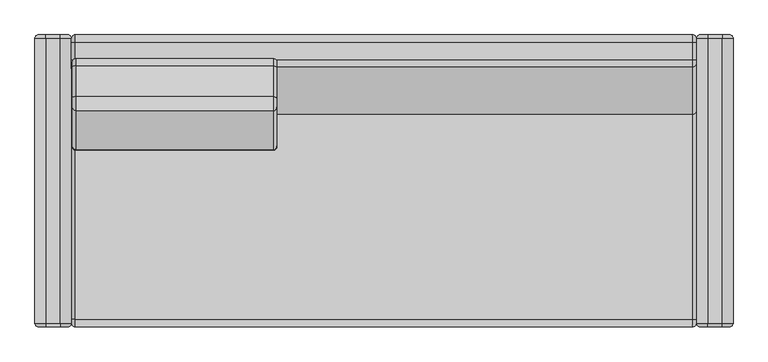
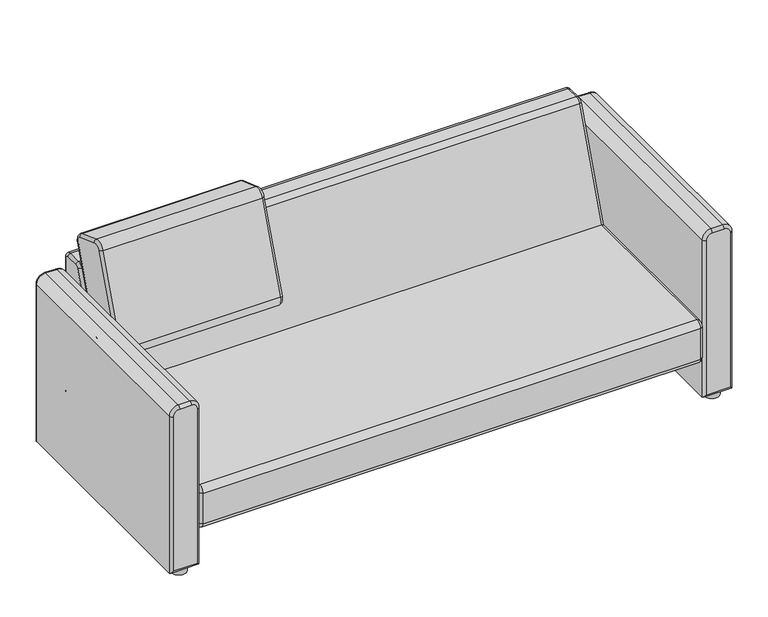
"""IFC4 building model written with IfcOpenShell, lengths in millimetres: furniture geometry."""

from ifc_helpers import new_model, si_unit, point, frame, frame_2d, origin, origin_with_axes, place, context, project, spatial, circle_curve, ellipse_curve, trimmed, segment, composite_curve, outline, extrude, source, transform, mapped, element, save
from ifc_brep_helpers import plane_surface, cylinder_surface, revolved_surface, advanced_brep


def furniture_2fc85b74(model_context):
    return source(origin(), model_context, "Body", "SolidModel", [
        advanced_brep(
        [(-945.0, 0.0, 590.0), (-945.0, 0.0, 35.0), (-865.0, 0.0, 35.0), (-865.0, 0.0, 590.0), (-885.0, 0.0, 610.0), (-925.0, 0.0, 610.0), (-865.0, 800.0, 590.0), (-865.0, 800.0, 35.0), (-945.0, 800.0, 35.0), (-945.0, 800.0, 590.0), (-925.0, 800.0, 610.0), (-885.0, 800.0, 610.0), (-855.0, 9.9999877, 590.0), (-855.0, 790.0000093, 590.0), (-885.0, 790.0, 620.0), (-885.0, 10.0, 620.0), (-925.0, 9.9999878, 620.0), (-925.0, 790.0, 620.0), (-955.0, 790.0, 590.0), (-955.0, 9.9999878, 590.0), (-855.0, 10.0, 25.0), (-855.0, 790.0, 25.0), (-955.0, 10.0, 25.0), (-955.0, 790.0, 25.0)],
        [
            (0, 1),
            (1, 2),
            (2, 3),
            (3, 4, circle_curve(frame((-885.0, 0.0, 590.0), z_axis=(0.0, -1.0, 0.0), x_axis=(0.0, 0.0, 1.0)), 20.0)),
            (4, 5),
            (5, 0, circle_curve(frame((-925.0, 0.0, 590.0), z_axis=(0.0, -1.0, 0.0), x_axis=(-1.0, 0.0, 0.0)), 20.0)),
            (6, 7),
            (7, 8),
            (8, 9),
            (9, 10, circle_curve(frame((-925.0, 800.0, 590.0), z_axis=(0.0, 1.0, 0.0), x_axis=(0.0, 0.0, 1.0)), 20.0)),
            (10, 11),
            (11, 6, circle_curve(frame((-885.0, 800.0, 590.0), z_axis=(0.0, 1.0, 0.0), x_axis=(1.0, 0.0, 0.0)), 20.0)),
            (12, 13),
            (13, 14, circle_curve(frame((-885.0, 790.0, 590.0), z_axis=(0.0, -1.0, 0.0), x_axis=(-1.0, 0.0, 0.0)), 30.0)),
            (14, 15),
            (15, 12, circle_curve(frame((-885.0, 10.0, 590.0), z_axis=(0.0, 1.0, 0.0), x_axis=(-1.0, 0.0, 0.0)), 30.0)),
            (16, 17),
            (17, 18, circle_curve(frame((-925.0, 790.0, 590.0), z_axis=(0.0, -1.0, 0.0), x_axis=(-1.0, 0.0, 0.0)), 30.0)),
            (18, 19),
            (19, 16, circle_curve(frame((-925.0, 10.0, 590.0), z_axis=(0.0, 1.0, 0.0), x_axis=(-1.0, 0.0, 0.0)), 30.0)),
            (20, 21),
            (21, 13),
            (12, 20),
            (22, 23),
            (23, 21),
            (20, 22),
            (18, 23),
            (22, 19),
            (14, 17),
            (16, 15),
            (19, 0, circle_curve(frame((-945.0, 10.0, 590.0), z_axis=(0.0, 0.0, 1.0), x_axis=(-1.0, 0.0, 0.0)), 10.0)),
            (5, 16, circle_curve(frame((-925.0, 10.0, 610.0), z_axis=(-1.0, 0.0, 0.0), x_axis=(0.0, 0.0, 1.0)), 10.0)),
            (4, 15, circle_curve(frame((-885.0, 10.0, 610.0), z_axis=(-1.0, 0.0, 0.0), x_axis=(0.0, 0.0, 1.0)), 10.0)),
            (3, 12, circle_curve(frame((-865.0, 10.0, 590.0), z_axis=(0.0, 0.0, 1.0), x_axis=(1.0, 0.0, 0.0)), 10.0)),
            (2, 20, ellipse_curve(frame((-865.0, 10.0, 35.0), z_axis=(0.7071067811865458, 0.0, 0.7071067811865492), x_axis=(0.7071067811865492, 0.0, -0.7071067811865458)), 14.1421356, 10.0)),
            (1, 22, ellipse_curve(frame((-945.0, 10.0, 35.0), z_axis=(0.7071067811865492, 0.0, -0.7071067811865457), x_axis=(-0.707106781186546, 0.0, -0.7071067811865491)), 14.1421356, 10.0)),
            (13, 6, circle_curve(frame((-865.0, 790.0, 590.0), z_axis=(0.0, 0.0, 1.0), x_axis=(-1.0, 0.0, 0.0)), 10.0)),
            (11, 14, circle_curve(frame((-885.0, 790.0, 610.0), z_axis=(1.0, 0.0, 0.0), x_axis=(0.0, 0.0, -1.0)), 10.0)),
            (10, 17, circle_curve(frame((-925.0, 790.0, 610.0), z_axis=(1.0, 0.0, 0.0), x_axis=(0.0, 0.0, -1.0)), 10.0)),
            (9, 18, circle_curve(frame((-945.0, 790.0, 590.0), z_axis=(0.0, 0.0, 1.0), x_axis=(1.0, 0.0, 0.0)), 10.0)),
            (8, 23, ellipse_curve(frame((-945.0, 790.0, 35.0), z_axis=(-0.7071067811865492, 0.0, 0.7071067811865458), x_axis=(-0.7071067811865457, 0.0, -0.7071067811865492)), 14.1421356, 10.0)),
            (7, 21, ellipse_curve(frame((-865.0, 790.0, 35.0), z_axis=(-0.707106781186546, 0.0, -0.7071067811865491), x_axis=(0.707106781186549, 0.0, -0.707106781186546)), 14.1421356, 10.0)),
        ],
        [
            plane_surface(frame((-915.0, 0.0, 590.0), z_axis=(0.0, -1.0, 0.0), x_axis=(0.0, 0.0, 1.0))),
            plane_surface(frame((-915.0, 800.0, 590.0), z_axis=(0.0, 1.0, 0.0), x_axis=(0.0, 0.0, -1.0))),
            cylinder_surface(frame((-885.0, 800.0, 590.0), z_axis=(0.0, -1.0, 0.0), x_axis=(-1.0, 0.0, 0.0)), 30.0),
            cylinder_surface(frame((-925.0, 800.0, 590.0), z_axis=(0.0, -1.0, 0.0), x_axis=(-1.0, 0.0, 0.0)), 30.0),
            plane_surface(frame((-855.0, 0.0, 590.0), z_axis=(1.0, 0.0, 0.0), x_axis=(0.0, 1.0, 0.0))),
            plane_surface(frame((-855.0, 0.0, 25.0), z_axis=(0.0, 0.0, -1.0), x_axis=(0.0, 1.0, 0.0))),
            plane_surface(frame((-955.0, 0.0, 25.0), z_axis=(-1.0, 0.0, 0.0), x_axis=(0.0, 1.0, 0.0))),
            plane_surface(frame((-925.0, 0.0, 620.0), z_axis=(0.0, 0.0, 1.0), x_axis=(0.0, 1.0, 0.0))),
            revolved_surface(trimmed(ellipse_curve(frame((-945.0, 10.0, 590.0), z_axis=(0.0, 0.0, 1.0), x_axis=(-1.0, 0.0, 0.0)), 10.0, 10.0), [point((-955.0, 10.0, 590.0))], [point((-945.0, 0.0, 590.0))], True, "CARTESIAN"), (-925.0, 0.0, 590.0), (0.0, -1.0, 0.0)),
            cylinder_surface(frame((-925.0, 10.0, 610.0), z_axis=(1.0, 0.0, 0.0), x_axis=(0.0, 0.0, 1.0)), 10.0),
            revolved_surface(trimmed(ellipse_curve(frame((-885.0, 10.0, 610.0), z_axis=(1.0, 0.0, 0.0), x_axis=(0.0, 0.0, 1.0)), 10.0, 10.0), [point((-885.0, 10.0, 620.0))], [point((-885.0, 0.0, 610.0))], True, "CARTESIAN"), (-885.0, 0.0, 590.0), (0.0, -1.0, 0.0)),
            cylinder_surface(frame((-865.0, 10.0, 590.0), z_axis=(0.0, 0.0, -1.0), x_axis=(1.0, 0.0, 0.0)), 10.0),
            cylinder_surface(frame((-855.0, 10.0, 35.0), z_axis=(-1.0, 0.0, 0.0), x_axis=(0.0, 0.0, -1.0)), 10.0),
            cylinder_surface(frame((-945.0, 10.0, 25.0), z_axis=(0.0, 0.0, 1.0), x_axis=(-1.0, 0.0, 0.0)), 10.0),
            revolved_surface(trimmed(ellipse_curve(frame((-865.0, 790.0, 590.0), z_axis=(0.0, 0.0, 1.0), x_axis=(-1.0, 0.0, 0.0)), 10.0, 10.0), [point((-855.0, 790.0, 590.0))], [point((-865.0, 800.0, 590.0))], True, "CARTESIAN"), (-885.0, 800.0, 590.0), (0.0, 1.0, 0.0)),
            cylinder_surface(frame((-885.0, 790.0, 610.0), z_axis=(-1.0, 0.0, 0.0), x_axis=(0.0, 0.0, -1.0)), 10.0),
            revolved_surface(trimmed(ellipse_curve(frame((-925.0, 790.0, 610.0), z_axis=(-1.0, 0.0, 0.0), x_axis=(0.0, 0.0, -1.0)), 10.0, 10.0), [point((-925.0, 790.0, 620.0))], [point((-925.0, 800.0, 610.0))], True, "CARTESIAN"), (-925.0, 800.0, 590.0), (0.0, 1.0, 0.0)),
            cylinder_surface(frame((-945.0, 790.0, 590.0), z_axis=(0.0, 0.0, -1.0), x_axis=(1.0, 0.0, 0.0)), 10.0),
            cylinder_surface(frame((-955.0, 790.0, 35.0), z_axis=(1.0, 0.0, 0.0), x_axis=(0.0, 0.0, 1.0)), 10.0),
            cylinder_surface(frame((-865.0, 790.0, 25.0), z_axis=(0.0, 0.0, 1.0), x_axis=(-1.0, 0.0, 0.0)), 10.0),
        ],
        [
            (0, [[1, 2, 3, 4, 5, 6]]),
            (1, [[7, 8, 9, 10, 11, 12]]),
            (2, [[13, 14, 15, 16]]),
            (3, [[17, 18, 19, 20]]),
            (4, [[21, 22, -13, 23]]),
            (5, [[24, 25, -21, 26]]),
            (6, [[-19, 27, -24, 28]]),
            (7, [[-15, 29, -17, 30]]),
            (8, [[-20, 31, -6, 32]]),
            (9, [[-5, 33, -30, -32]]),
            (10, [[-4, 34, -16, -33]]),
            (11, [[-3, 35, -23, -34]]),
            (12, [[-2, 36, -26, -35]]),
            (13, [[-28, -36, -1, -31]]),
            (14, [[-14, 37, -12, 38]]),
            (15, [[-11, 39, -29, -38]]),
            (16, [[-10, 40, -18, -39]]),
            (17, [[-9, 41, -27, -40]]),
            (18, [[-8, 42, -25, -41]]),
            (19, [[-22, -42, -7, -37]]),
        ],
    ),
        extrude(outline(composite_curve([segment(trimmed(circle_curve(frame_2d((-905.0, 760.0)), 25.0), [point((-880.0, 760.0))], [point((-930.0, 760.0))], False, "CARTESIAN"), True, "CONTINUOUS"), segment(trimmed(circle_curve(frame_2d((-905.0, 760.0)), 25.0), [point((-930.0, 760.0))], [point((-880.0, 760.0))], False, "CARTESIAN"), True, "CONTINUOUS")], self_intersect=False)), origin_with_axes(), (0.0, 0.0, 1.0), 25.0),
        extrude(outline(composite_curve([segment(trimmed(circle_curve(frame_2d((-905.0, 40.0)), 25.0), [point((-880.0, 40.0))], [point((-930.0, 40.0))], False, "CARTESIAN"), True, "CONTINUOUS"), segment(trimmed(circle_curve(frame_2d((-905.0, 40.0)), 25.0), [point((-930.0, 40.0))], [point((-880.0, 40.0))], False, "CARTESIAN"), True, "CONTINUOUS")], self_intersect=False)), origin_with_axes(), (0.0, 0.0, 1.0), 25.0),
        advanced_brep(
        [(946.1853865, 0.0, 590.0), (926.1853865, 0.0, 610.0), (886.1853865, 0.0, 610.0), (866.1853865, 0.0, 590.0), (866.1853865, 0.0, 35.0), (946.1853865, 0.0, 35.0), (866.1853865, 800.0, 590.0), (886.1853865, 800.0, 610.0), (926.1853865, 800.0, 610.0), (946.1853865, 800.0, 590.0), (946.1853865, 800.0, 35.0), (866.1853865, 800.0, 35.0), (856.1853865, 10.0, 590.0), (886.1853865, 10.0, 620.0), (886.1853865, 790.000012, 620.0), (856.1853865, 790.0, 590.0), (926.1853865, 10.0, 620.0), (956.1853865, 10.0, 590.0), (956.1853865, 790.0000092, 590.0), (926.1853865, 790.0, 620.0), (856.1853865, 10.0, 25.0), (856.1853865, 790.0, 25.0), (956.1853865, 10.0, 25.0), (956.1853865, 790.0, 25.0)],
        [
            (0, 1, circle_curve(frame((926.1853865, 0.0, 590.0), z_axis=(0.0, -1.0, 0.0), x_axis=(1.0, 0.0, 0.0)), 20.0)),
            (1, 2),
            (2, 3, circle_curve(frame((886.1853865, 0.0, 590.0), z_axis=(0.0, -1.0, 0.0), x_axis=(0.0, 0.0, 1.0)), 20.0)),
            (3, 4),
            (4, 5),
            (5, 0),
            (6, 7, circle_curve(frame((886.1853865, 800.0, 590.0), z_axis=(0.0, 1.0, 0.0), x_axis=(-1.0, 0.0, 0.0)), 20.0)),
            (7, 8),
            (8, 9, circle_curve(frame((926.1853865, 800.0, 590.0), z_axis=(0.0, 1.0, 0.0), x_axis=(0.0, 0.0, 1.0)), 20.0)),
            (9, 10),
            (10, 11),
            (11, 6),
            (12, 13, circle_curve(frame((886.1853865, 10.0, 590.0), z_axis=(0.0, 1.0, 0.0), x_axis=(1.0, 0.0, 0.0)), 30.0)),
            (13, 14),
            (14, 15, circle_curve(frame((886.1853865, 790.0, 590.0), z_axis=(0.0, -1.0, 0.0), x_axis=(1.0, 0.0, 0.0)), 30.0)),
            (15, 12),
            (16, 17, circle_curve(frame((926.1853865, 10.0, 590.0), z_axis=(0.0, 1.0, 0.0), x_axis=(1.0, 0.0, 0.0)), 30.0)),
            (17, 18),
            (18, 19, circle_curve(frame((926.1853865, 790.0, 590.0), z_axis=(0.0, -1.0, 0.0), x_axis=(1.0, 0.0, 0.0)), 30.0)),
            (19, 16),
            (20, 12),
            (15, 21),
            (21, 20),
            (22, 20),
            (21, 23),
            (23, 22),
            (17, 22),
            (23, 18),
            (13, 16),
            (19, 14),
            (16, 1, circle_curve(frame((926.1853865, 10.0, 610.0), z_axis=(1.0, 0.0, 0.0), x_axis=(0.0, 0.0, 1.0)), 10.0)),
            (0, 17, circle_curve(frame((946.1853865, 10.0, 590.0), z_axis=(0.0, 0.0, 1.0), x_axis=(1.0, 0.0, 0.0)), 10.0)),
            (13, 2, circle_curve(frame((886.1853865, 10.0, 610.0), z_axis=(1.0, 0.0, 0.0), x_axis=(0.0, 0.0, 1.0)), 10.0)),
            (12, 3, circle_curve(frame((866.1853865, 10.0, 590.0), z_axis=(0.0, 0.0, 1.0), x_axis=(-1.0, 0.0, 0.0)), 10.0)),
            (20, 4, ellipse_curve(frame((866.1853865, 10.0, 35.0), z_axis=(-0.7071067811865458, 0.0, 0.7071067811865492), x_axis=(-0.7071067811865492, 0.0, -0.7071067811865458)), 14.1421356, 10.0)),
            (22, 5, ellipse_curve(frame((946.1853865, 10.0, 35.0), z_axis=(-0.7071067811865492, 0.0, -0.7071067811865457), x_axis=(0.707106781186546, 0.0, -0.7071067811865491)), 14.1421356, 10.0)),
            (14, 7, circle_curve(frame((886.1853865, 790.0, 610.0), z_axis=(-1.0, 0.0, 0.0), x_axis=(0.0, 0.0, -1.0)), 10.0)),
            (6, 15, circle_curve(frame((866.1853865, 790.0, 590.0), z_axis=(0.0, 0.0, 1.0), x_axis=(1.0, 0.0, 0.0)), 10.0)),
            (19, 8, circle_curve(frame((926.1853865, 790.0, 610.0), z_axis=(-1.0, 0.0, 0.0), x_axis=(0.0, 0.0, -1.0)), 10.0)),
            (18, 9, circle_curve(frame((946.1853865, 790.0, 590.0), z_axis=(0.0, 0.0, 1.0), x_axis=(-1.0, 0.0, 0.0)), 10.0)),
            (23, 10, ellipse_curve(frame((946.1853865, 790.0, 35.0), z_axis=(0.7071067811865492, 0.0, 0.7071067811865458), x_axis=(0.7071067811865457, 0.0, -0.7071067811865492)), 14.1421356, 10.0)),
            (21, 11, ellipse_curve(frame((866.1853865, 790.0, 35.0), z_axis=(0.707106781186546, 0.0, -0.7071067811865491), x_axis=(-0.707106781186549, 0.0, -0.707106781186546)), 14.1421356, 10.0)),
        ],
        [
            plane_surface(frame((916.1853865, 0.0, 590.0), z_axis=(0.0, -1.0, 0.0), x_axis=(0.0, 0.0, 1.0))),
            plane_surface(frame((916.1853865, 800.0, 590.0), z_axis=(0.0, 1.0, 0.0), x_axis=(0.0, 0.0, -1.0))),
            cylinder_surface(frame((886.1853865, 800.0, 590.0), z_axis=(0.0, -1.0, 0.0), x_axis=(1.0, 0.0, 0.0)), 30.0),
            cylinder_surface(frame((926.1853865, 800.0, 590.0), z_axis=(0.0, -1.0, 0.0), x_axis=(1.0, 0.0, 0.0)), 30.0),
            plane_surface(frame((856.1853865, 0.0, 590.0), z_axis=(-1.0, 0.0, 0.0), x_axis=(0.0, 1.0, 0.0))),
            plane_surface(frame((856.1853865, 0.0, 25.0), z_axis=(0.0, 0.0, -1.0), x_axis=(0.0, 1.0, 0.0))),
            plane_surface(frame((956.1853865, 0.0, 25.0), z_axis=(1.0, 0.0, 0.0), x_axis=(0.0, 1.0, 0.0))),
            plane_surface(frame((926.1853865, 0.0, 620.0), z_axis=(0.0, 0.0, 1.0), x_axis=(0.0, 1.0, 0.0))),
            revolved_surface(trimmed(ellipse_curve(frame((946.1853865, 10.0, 590.0), z_axis=(0.0, 0.0, -1.0), x_axis=(1.0, 0.0, 0.0)), 10.0, 10.0), [point((956.1853865, 10.0, 590.0))], [point((946.1853865, 0.0, 590.0))], True, "CARTESIAN"), (926.1853865, 0.0, 590.0), (0.0, -1.0, 0.0)),
            cylinder_surface(frame((926.1853865, 10.0, 610.0), z_axis=(-1.0, 0.0, 0.0), x_axis=(0.0, 0.0, 1.0)), 10.0),
            revolved_surface(trimmed(ellipse_curve(frame((886.1853865, 10.0, 610.0), z_axis=(1.0, 0.0, 0.0), x_axis=(0.0, 0.0, 1.0)), 10.0, 10.0), [point((886.1853865, 10.0, 620.0))], [point((886.1853865, 0.0, 610.0))], True, "CARTESIAN"), (886.1853865, 0.0, 590.0), (0.0, -1.0, 0.0)),
            cylinder_surface(frame((866.1853865, 10.0, 590.0), z_axis=(0.0, 0.0, -1.0), x_axis=(-1.0, 0.0, 0.0)), 10.0),
            cylinder_surface(frame((856.1853865, 10.0, 35.0), z_axis=(1.0, 0.0, 0.0), x_axis=(0.0, 0.0, -1.0)), 10.0),
            cylinder_surface(frame((946.1853865, 10.0, 25.0), z_axis=(0.0, 0.0, 1.0), x_axis=(1.0, 0.0, 0.0)), 10.0),
            revolved_surface(trimmed(ellipse_curve(frame((866.1853865, 790.0, 590.0), z_axis=(0.0, 0.0, -1.0), x_axis=(1.0, 0.0, 0.0)), 10.0, 10.0), [point((856.1853865, 790.0, 590.0))], [point((866.1853865, 800.0, 590.0))], True, "CARTESIAN"), (886.1853865, 800.0, 590.0), (0.0, 1.0, 0.0)),
            cylinder_surface(frame((886.1853865, 790.0, 610.0), z_axis=(1.0, 0.0, 0.0), x_axis=(0.0, 0.0, -1.0)), 10.0),
            revolved_surface(trimmed(ellipse_curve(frame((926.1853865, 790.0, 610.0), z_axis=(-1.0, 0.0, 0.0), x_axis=(0.0, 0.0, -1.0)), 10.0, 10.0), [point((926.1853865, 790.0, 620.0))], [point((926.1853865, 800.0, 610.0))], True, "CARTESIAN"), (926.1853865, 800.0, 590.0), (0.0, 1.0, 0.0)),
            cylinder_surface(frame((946.1853865, 790.0, 590.0), z_axis=(0.0, 0.0, -1.0), x_axis=(-1.0, 0.0, 0.0)), 10.0),
            cylinder_surface(frame((956.1853865, 790.0, 35.0), z_axis=(-1.0, 0.0, 0.0), x_axis=(0.0, 0.0, 1.0)), 10.0),
            cylinder_surface(frame((866.1853865, 790.0, 25.0), z_axis=(0.0, 0.0, 1.0), x_axis=(1.0, 0.0, 0.0)), 10.0),
        ],
        [
            (0, [[1, 2, 3, 4, 5, 6]]),
            (1, [[7, 8, 9, 10, 11, 12]]),
            (2, [[13, 14, 15, 16]]),
            (3, [[17, 18, 19, 20]]),
            (4, [[21, -16, 22, 23]]),
            (5, [[24, -23, 25, 26]]),
            (6, [[27, -26, 28, -18]]),
            (7, [[29, -20, 30, -14]]),
            (8, [[31, -1, 32, -17]]),
            (9, [[-31, -29, 33, -2]]),
            (10, [[-33, -13, 34, -3]]),
            (11, [[-34, -21, 35, -4]]),
            (12, [[-35, -24, 36, -5]]),
            (13, [[-32, -6, -36, -27]]),
            (14, [[37, -7, 38, -15]]),
            (15, [[-37, -30, 39, -8]]),
            (16, [[-39, -19, 40, -9]]),
            (17, [[-40, -28, 41, -10]]),
            (18, [[-41, -25, 42, -11]]),
            (19, [[-38, -12, -42, -22]]),
        ],
    ),
        extrude(outline(composite_curve([segment(trimmed(circle_curve(frame_2d((906.1853865, 760.0)), 25.0), [point((881.1853865, 760.0))], [point((931.1853865, 760.0))], False, "CARTESIAN"), True, "CONTINUOUS"), segment(trimmed(circle_curve(frame_2d((906.1853865, 760.0)), 25.0), [point((931.1853865, 760.0))], [point((881.1853865, 760.0))], False, "CARTESIAN"), True, "CONTINUOUS")], self_intersect=False)), origin_with_axes(), (0.0, 0.0, 1.0), 25.0),
        extrude(outline(composite_curve([segment(trimmed(circle_curve(frame_2d((906.1853865, 40.0)), 25.0), [point((881.1853865, 40.0))], [point((931.1853865, 40.0))], False, "CARTESIAN"), True, "CONTINUOUS"), segment(trimmed(circle_curve(frame_2d((906.1853865, 40.0)), 25.0), [point((931.1853865, 40.0))], [point((881.1853865, 40.0))], False, "CARTESIAN"), True, "CONTINUOUS")], self_intersect=False)), origin_with_axes(), (0.0, 0.0, 1.0), 25.0),
        advanced_brep(
        [(855.0, 731.2835554, 660.0), (855.0, 721.8866292, 653.4202014), (855.0, 589.6124934, 290.0), (855.0, 20.0, 290.0), (855.0, 10.0, 280.0), (855.0, 10.0, 170.0), (855.0, 20.0, 160.0), (855.0, 780.0, 160.0), (855.0, 790.0, 170.0), (855.0, 790.0, 650.0), (855.0, 780.0, 660.0), (-855.0, 780.0, 660.0), (-855.0, 790.0, 650.0), (-855.0, 790.0, 170.0), (-855.0, 780.0, 160.0), (-855.0, 20.0, 160.0), (-855.0, 10.0, 170.0), (-855.0, 10.0, 280.0), (-855.0, 20.0, 290.0), (-855.0, 589.6124934, 290.0), (-855.0, 721.8866292, 653.4202014), (-855.0, 731.2835554, 660.0), (-845.0, 731.2835554, 670.0), (-845.0, 712.489703, 656.8404029), (845.0000088, 712.489703, 656.8404029), (845.0, 731.2835554, 670.0), (-845.0, 582.610418, 300.0), (845.0, 582.610418, 300.0), (-845.0, 20.0, 300.0), (845.0, 20.0, 300.0), (-845.0, 0.0, 280.0), (845.000009, 0.0, 280.0), (-845.0, 0.0, 170.0), (845.0, 0.0, 170.0), (-845.0, 20.0, 150.0), (845.000009, 20.0, 150.0), (-845.0, 780.0, 150.0), (845.0, 780.0, 150.0), (-845.0, 800.0, 170.0), (845.000009, 800.0, 170.0), (-845.0, 800.0, 650.0), (845.0, 800.0, 650.0), (-845.0, 780.0, 670.0), (845.0000092, 780.0, 670.0)],
        [
            (0, 1, circle_curve(frame((855.0, 731.2835554, 650.0), z_axis=(1.0, 0.0, 0.0), x_axis=(0.0, 0.0, 1.0)), 10.0)),
            (1, 2),
            (2, 3),
            (3, 4, circle_curve(frame((855.0, 20.0, 280.0), z_axis=(1.0, 0.0, 0.0), x_axis=(0.0, 0.0, 1.0)), 10.0)),
            (4, 5),
            (5, 6, circle_curve(frame((855.0, 20.0, 170.0), z_axis=(1.0, 0.0, 0.0), x_axis=(0.0, -1.0, 0.0)), 10.0)),
            (6, 7),
            (7, 8, circle_curve(frame((855.0, 780.0, 170.0), z_axis=(1.0, 0.0, 0.0), x_axis=(0.0, 0.0, -1.0)), 10.0)),
            (8, 9),
            (9, 10, circle_curve(frame((855.0, 780.0, 650.0), z_axis=(1.0, 0.0, 0.0), x_axis=(0.0, 1.0, 0.0)), 10.0)),
            (10, 0),
            (11, 12, circle_curve(frame((-855.0, 780.0, 650.0), z_axis=(-1.0, 0.0, 0.0), x_axis=(0.0, 0.0, 1.0)), 10.0)),
            (12, 13),
            (13, 14, circle_curve(frame((-855.0, 780.0, 170.0), z_axis=(-1.0, 0.0, 0.0), x_axis=(0.0, 1.0, 0.0)), 10.0)),
            (14, 15),
            (15, 16, circle_curve(frame((-855.0, 20.0, 170.0), z_axis=(-1.0, 0.0, 0.0), x_axis=(0.0, 0.0, -1.0)), 10.0)),
            (16, 17),
            (17, 18, circle_curve(frame((-855.0, 20.0, 280.0), z_axis=(-1.0, 0.0, 0.0), x_axis=(0.0, -1.0, 0.0)), 10.0)),
            (18, 19),
            (19, 20),
            (20, 21, circle_curve(frame((-855.0, 731.2835554, 650.0), z_axis=(-1.0, 0.0, 0.0), x_axis=(0.0, -0.9396926207859069, 0.3420201433256728)), 10.0)),
            (21, 11),
            (22, 23, circle_curve(frame((-845.0, 731.2835554, 650.0), z_axis=(1.0, 0.0, 0.0), x_axis=(0.0, 1.0, 0.0)), 20.0)),
            (23, 24),
            (24, 25, circle_curve(frame((845.0, 731.2835554, 650.0), z_axis=(-1.0, 0.0, 0.0), x_axis=(0.0, 1.0, 0.0)), 20.0)),
            (25, 22),
            (23, 26),
            (26, 27),
            (27, 24),
            (26, 28),
            (28, 29),
            (29, 27),
            (28, 30, circle_curve(frame((-845.0, 20.0, 280.0), z_axis=(1.0, 0.0, 0.0), x_axis=(0.0, 1.0, 0.0)), 20.0)),
            (30, 31),
            (31, 29, circle_curve(frame((845.0, 20.0, 280.0), z_axis=(-1.0, 0.0, 0.0), x_axis=(0.0, 1.0, 0.0)), 20.0)),
            (30, 32),
            (32, 33),
            (33, 31),
            (32, 34, circle_curve(frame((-845.0, 20.0, 170.0), z_axis=(1.0, 0.0, 0.0), x_axis=(0.0, 1.0, 0.0)), 20.0)),
            (34, 35),
            (35, 33, circle_curve(frame((845.0, 20.0, 170.0), z_axis=(-1.0, 0.0, 0.0), x_axis=(0.0, 1.0, 0.0)), 20.0)),
            (34, 36),
            (36, 37),
            (37, 35),
            (36, 38, circle_curve(frame((-845.0, 780.0, 170.0), z_axis=(1.0, 0.0, 0.0), x_axis=(0.0, 1.0, 0.0)), 20.0)),
            (38, 39),
            (39, 37, circle_curve(frame((845.0, 780.0, 170.0), z_axis=(-1.0, 0.0, 0.0), x_axis=(0.0, 1.0, 0.0)), 20.0)),
            (38, 40),
            (40, 41),
            (41, 39),
            (40, 42, circle_curve(frame((-845.0, 780.0, 650.0), z_axis=(1.0, 0.0, 0.0), x_axis=(0.0, 1.0, 0.0)), 20.0)),
            (42, 43),
            (43, 41, circle_curve(frame((845.0, 780.0, 650.0), z_axis=(-1.0, 0.0, 0.0), x_axis=(0.0, 1.0, 0.0)), 20.0)),
            (42, 22),
            (25, 43),
            (40, 12, circle_curve(frame((-845.0, 790.0, 650.0), z_axis=(0.0, 0.0, 1.0), x_axis=(-1.0, 0.0, 0.0)), 10.0)),
            (11, 42, circle_curve(frame((-845.0, 780.0, 660.0), z_axis=(0.0, 1.0, 0.0), x_axis=(-1.0, 0.0, 0.0)), 10.0)),
            (38, 13, circle_curve(frame((-845.0, 790.0, 170.0), z_axis=(0.0, 0.0, 1.0), x_axis=(-1.0, 0.0, 0.0)), 10.0)),
            (36, 14, circle_curve(frame((-845.0, 780.0, 160.0), z_axis=(0.0, 1.0, 0.0), x_axis=(-1.0, 0.0, 0.0)), 10.0)),
            (34, 15, circle_curve(frame((-845.0, 20.0, 160.0), z_axis=(0.0, 1.0, 0.0), x_axis=(-1.0, 0.0, 0.0)), 10.0)),
            (32, 16, circle_curve(frame((-845.0, 10.0, 170.0), z_axis=(0.0, 0.0, -1.0), x_axis=(-1.0, 0.0, 0.0)), 10.0)),
            (30, 17, circle_curve(frame((-845.0, 10.0, 280.0), z_axis=(0.0, 0.0, -1.0), x_axis=(-1.0, 0.0, 0.0)), 10.0)),
            (28, 18, circle_curve(frame((-845.0, 20.0, 290.0), z_axis=(0.0, -1.0, 0.0), x_axis=(-1.0, 0.0, 0.0)), 10.0)),
            (26, 19, ellipse_curve(frame((-845.0, 589.6124934, 290.0), z_axis=(0.0, -0.8191520442889938, -0.573576436351043), x_axis=(0.0, 0.5735764363510434, -0.8191520442889938)), 12.2077459, 10.0)),
            (23, 20, circle_curve(frame((-845.0, 721.8866292, 653.4202014), z_axis=(0.0, -0.34202014332567243, -0.9396926207859071), x_axis=(-1.0, 0.0, 0.0)), 10.0)),
            (22, 21, circle_curve(frame((-845.0, 731.2835554, 660.0), z_axis=(0.0, -1.0, 0.0), x_axis=(-1.0, 0.0, 0.0)), 10.0)),
            (24, 1, circle_curve(frame((845.0, 721.8866292, 653.4202014), z_axis=(0.0, 0.3420201433256818, 0.9396926207859037), x_axis=(1.0, 0.0, 0.0)), 10.0)),
            (0, 25, circle_curve(frame((845.0, 731.2835554, 660.0), z_axis=(0.0, -1.0, 0.0), x_axis=(1.0, 0.0, 0.0)), 10.0)),
            (27, 2, ellipse_curve(frame((845.0, 589.6124934, 290.0), z_axis=(0.0, 0.8191520442889938, 0.5735764363510432), x_axis=(0.0, 0.5735764363510432, -0.8191520442889939)), 12.2077459, 10.0)),
            (29, 3, circle_curve(frame((845.0, 20.0, 290.0), z_axis=(0.0, 1.0, 0.0), x_axis=(1.0, 0.0, 0.0)), 10.0)),
            (31, 4, circle_curve(frame((845.0, 10.0, 280.0), z_axis=(0.0, 0.0, 1.0), x_axis=(1.0, 0.0, 0.0)), 10.0)),
            (33, 5, circle_curve(frame((845.0, 10.0, 170.0), z_axis=(0.0, 0.0, 1.0), x_axis=(1.0, 0.0, 0.0)), 10.0)),
            (35, 6, circle_curve(frame((845.0, 20.0, 160.0), z_axis=(0.0, -1.0, 0.0), x_axis=(1.0, 0.0, 0.0)), 10.0)),
            (37, 7, circle_curve(frame((845.0, 780.0, 160.0), z_axis=(0.0, -1.0, 0.0), x_axis=(1.0, 0.0, 0.0)), 10.0)),
            (39, 8, circle_curve(frame((845.0, 790.0, 170.0), z_axis=(0.0, 0.0, -1.0), x_axis=(1.0, 0.0, 0.0)), 10.0)),
            (41, 9, circle_curve(frame((845.0, 790.0, 650.0), z_axis=(0.0, 0.0, -1.0), x_axis=(1.0, 0.0, 0.0)), 10.0)),
            (43, 10, circle_curve(frame((845.0, 780.0, 660.0), z_axis=(0.0, 1.0, 0.0), x_axis=(1.0, 0.0, 0.0)), 10.0)),
        ],
        [
            plane_surface(frame((855.0, 751.2835554, 650.0), z_axis=(1.0, 0.0, 0.0), x_axis=(0.0, 0.0, 1.0))),
            plane_surface(frame((-855.0, 751.2835554, 650.0), z_axis=(-1.0, 0.0, 0.0), x_axis=(0.0, 0.0, -1.0))),
            cylinder_surface(frame((-855.0, 731.2835554, 650.0), z_axis=(1.0, 0.0, 0.0), x_axis=(0.0, 1.0, 0.0)), 20.0),
            plane_surface(frame((855.0, 712.489703, 656.8404029), z_axis=(0.0, -0.9396926207859071, 0.3420201433256725), x_axis=(-1.0, 0.0, 0.0))),
            plane_surface(frame((855.0, 582.610418, 300.0), z_axis=(0.0, 0.0, 1.0), x_axis=(-1.0, 0.0, 0.0))),
            cylinder_surface(frame((-855.0, 20.0, 280.0), z_axis=(1.0, 0.0, 0.0), x_axis=(0.0, 1.0, 0.0)), 20.0),
            plane_surface(frame((855.0, 0.0, 280.0), z_axis=(0.0, -1.0, 0.0), x_axis=(-1.0, 0.0, 0.0))),
            cylinder_surface(frame((-855.0, 20.0, 170.0), z_axis=(1.0, 0.0, 0.0), x_axis=(0.0, 1.0, 0.0)), 20.0),
            plane_surface(frame((855.0, 20.0, 150.0), z_axis=(0.0, 0.0, -1.0), x_axis=(-1.0, 0.0, 0.0))),
            cylinder_surface(frame((-855.0, 780.0, 170.0), z_axis=(1.0, 0.0, 0.0), x_axis=(0.0, 1.0, 0.0)), 20.0),
            plane_surface(frame((855.0, 800.0, 170.0), z_axis=(0.0, 1.0, 0.0), x_axis=(-1.0, 0.0, 0.0))),
            cylinder_surface(frame((-855.0, 780.0, 650.0), z_axis=(1.0, 0.0, 0.0), x_axis=(0.0, 1.0, 0.0)), 20.0),
            plane_surface(frame((855.0, 780.0, 670.0), z_axis=(0.0, 0.0, 1.0), x_axis=(-1.0, 0.0, 0.0))),
            revolved_surface(trimmed(ellipse_curve(frame((-845.0, 780.0, 660.0), z_axis=(0.0, -1.0, 0.0), x_axis=(-1.0, 0.0, 0.0)), 10.0, 10.0), [point((-845.0, 780.0, 670.0))], [point((-855.0, 780.0, 660.0))], True, "CARTESIAN"), (-855.0, 780.0, 650.0), (-1.0, 0.0, 0.0)),
            cylinder_surface(frame((-845.0, 790.0, 650.0), z_axis=(0.0, 0.0, -1.0), x_axis=(-1.0, 0.0, 0.0)), 10.0),
            revolved_surface(trimmed(ellipse_curve(frame((-845.0, 790.0, 170.0), z_axis=(0.0, 0.0, 1.0), x_axis=(-1.0, 0.0, 0.0)), 10.0, 10.0), [point((-845.0, 800.0, 170.0))], [point((-855.0, 790.0, 170.0))], True, "CARTESIAN"), (-855.0, 780.0, 170.0), (-1.0, 0.0, 0.0)),
            cylinder_surface(frame((-845.0, 780.0, 160.0), z_axis=(0.0, -1.0, 0.0), x_axis=(-1.0, 0.0, 0.0)), 10.0),
            revolved_surface(trimmed(ellipse_curve(frame((-845.0, 20.0, 160.0), z_axis=(0.0, 1.0, 0.0), x_axis=(-1.0, 0.0, 0.0)), 10.0, 10.0), [point((-845.0, 20.0, 150.0))], [point((-855.0, 20.0, 160.0))], True, "CARTESIAN"), (-855.0, 20.0, 170.0), (-1.0, 0.0, 0.0)),
            cylinder_surface(frame((-845.0, 10.0, 170.0), z_axis=(0.0, 0.0, 1.0), x_axis=(-1.0, 0.0, 0.0)), 10.0),
            revolved_surface(trimmed(ellipse_curve(frame((-845.0, 10.0, 280.0), z_axis=(0.0, 0.0, -1.0), x_axis=(-1.0, 0.0, 0.0)), 10.0, 10.0), [point((-845.0, 0.0, 280.0))], [point((-855.0, 10.0, 280.0))], True, "CARTESIAN"), (-855.0, 20.0, 280.0), (-1.0, 0.0, 0.0)),
            cylinder_surface(frame((-845.0, 20.0, 290.0), z_axis=(0.0, 1.0, 0.0), x_axis=(-1.0, 0.0, 0.0)), 10.0),
            cylinder_surface(frame((-845.0, 592.0073442, 296.5797986), z_axis=(0.0, 0.34202014332567243, 0.9396926207859071), x_axis=(-1.0, 0.0, 0.0)), 10.0),
            revolved_surface(trimmed(ellipse_curve(frame((-845.0, 721.8866292, 653.4202014), z_axis=(0.0, -0.3420201433256728, -0.9396926207859069), x_axis=(-1.0, 0.0, 0.0)), 10.0, 10.0), [point((-845.0, 712.489703, 656.8404029))], [point((-855.0, 721.8866292, 653.4202014))], True, "CARTESIAN"), (-855.0, 731.2835554, 650.0), (-1.0, 0.0, 0.0)),
            cylinder_surface(frame((-845.0, 731.2835554, 660.0), z_axis=(0.0, 1.0, 0.0), x_axis=(-1.0, 0.0, 0.0)), 10.0),
            revolved_surface(trimmed(ellipse_curve(frame((845.0, 731.2835554, 660.0), z_axis=(0.0, 1.0, 0.0), x_axis=(1.0, 0.0, 0.0)), 10.0, 10.0), [point((845.0, 731.2835554, 670.0))], [point((855.0, 731.2835554, 660.0))], True, "CARTESIAN"), (855.0, 731.2835554, 650.0), (1.0, 0.0, 0.0)),
            cylinder_surface(frame((845.0, 721.8866292, 653.4202014), z_axis=(0.0, -0.34202014332567243, -0.9396926207859071), x_axis=(1.0, 0.0, 0.0)), 10.0),
            cylinder_surface(frame((845.0, 582.610418, 290.0), z_axis=(0.0, -1.0, 0.0), x_axis=(1.0, 0.0, 0.0)), 10.0),
            revolved_surface(trimmed(ellipse_curve(frame((845.0, 20.0, 290.0), z_axis=(0.0, 1.0, 0.0), x_axis=(1.0, 0.0, 0.0)), 10.0, 10.0), [point((845.0, 20.0, 300.0))], [point((855.0, 20.0, 290.0))], True, "CARTESIAN"), (855.0, 20.0, 280.0), (1.0, 0.0, 0.0)),
            cylinder_surface(frame((845.0, 10.0, 280.0), z_axis=(0.0, 0.0, -1.0), x_axis=(1.0, 0.0, 0.0)), 10.0),
            revolved_surface(trimmed(ellipse_curve(frame((845.0, 10.0, 170.0), z_axis=(0.0, 0.0, 1.0), x_axis=(1.0, 0.0, 0.0)), 10.0, 10.0), [point((845.0, 0.0, 170.0))], [point((855.0, 10.0, 170.0))], True, "CARTESIAN"), (855.0, 20.0, 170.0), (1.0, 0.0, 0.0)),
            cylinder_surface(frame((845.0, 20.0, 160.0), z_axis=(0.0, 1.0, 0.0), x_axis=(1.0, 0.0, 0.0)), 10.0),
            revolved_surface(trimmed(ellipse_curve(frame((845.0, 780.0, 160.0), z_axis=(0.0, -1.0, 0.0), x_axis=(1.0, 0.0, 0.0)), 10.0, 10.0), [point((845.0, 780.0, 150.0))], [point((855.0, 780.0, 160.0))], True, "CARTESIAN"), (855.0, 780.0, 170.0), (1.0, 0.0, 0.0)),
            cylinder_surface(frame((845.0, 790.0, 170.0), z_axis=(0.0, 0.0, 1.0), x_axis=(1.0, 0.0, 0.0)), 10.0),
            revolved_surface(trimmed(ellipse_curve(frame((845.0, 790.0, 650.0), z_axis=(0.0, 0.0, -1.0), x_axis=(1.0, 0.0, 0.0)), 10.0, 10.0), [point((845.0, 800.0, 650.0))], [point((855.0, 790.0, 650.0))], True, "CARTESIAN"), (855.0, 780.0, 650.0), (1.0, 0.0, 0.0)),
            cylinder_surface(frame((845.0, 780.0, 660.0), z_axis=(0.0, -1.0, 0.0), x_axis=(1.0, 0.0, 0.0)), 10.0),
        ],
        [
            (0, [[1, 2, 3, 4, 5, 6, 7, 8, 9, 10, 11]]),
            (1, [[12, 13, 14, 15, 16, 17, 18, 19, 20, 21, 22]]),
            (2, [[23, 24, 25, 26]]),
            (3, [[27, 28, 29, -24]]),
            (4, [[30, 31, 32, -28]]),
            (5, [[33, 34, 35, -31]]),
            (6, [[36, 37, 38, -34]]),
            (7, [[39, 40, 41, -37]]),
            (8, [[42, 43, 44, -40]]),
            (9, [[45, 46, 47, -43]]),
            (10, [[48, 49, 50, -46]]),
            (11, [[51, 52, 53, -49]]),
            (12, [[54, -26, 55, -52]]),
            (13, [[56, -12, 57, -51]]),
            (14, [[-56, -48, 58, -13]]),
            (15, [[-58, -45, 59, -14]]),
            (16, [[-59, -42, 60, -15]]),
            (17, [[-60, -39, 61, -16]]),
            (18, [[-61, -36, 62, -17]]),
            (19, [[-62, -33, 63, -18]]),
            (20, [[-63, -30, 64, -19]]),
            (21, [[-64, -27, 65, -20]]),
            (22, [[-65, -23, 66, -21]]),
            (23, [[-57, -22, -66, -54]]),
            (24, [[67, -1, 68, -25]]),
            (25, [[-67, -29, 69, -2]]),
            (26, [[-69, -32, 70, -3]]),
            (27, [[-70, -35, 71, -4]]),
            (28, [[-71, -38, 72, -5]]),
            (29, [[-72, -41, 73, -6]]),
            (30, [[-73, -44, 74, -7]]),
            (31, [[-74, -47, 75, -8]]),
            (32, [[-75, -50, 76, -9]]),
            (33, [[-76, -53, 77, -10]]),
            (34, [[-68, -11, -77, -55]]),
        ],
    ),
        advanced_brep(
        [(-292.5, 609.5185405, 469.9348489), (-292.5, 628.3736149, 483.1373142), (-292.5, 723.5847628, 744.7277933), (-292.5, 711.5923743, 770.4455535), (-292.5, 627.0200384, 801.2273664), (-292.5, 601.3022782, 789.2349779), (-292.5, 494.8874666, 496.8626858), (-292.5, 513.742541, 469.9348489), (-852.5, 513.742541, 469.9348489), (-852.5, 494.8874666, 496.8626858), (-852.5, 601.3022782, 789.2349779), (-852.5, 627.0200384, 801.2273664), (-852.5, 711.5923743, 770.4455535), (-852.5, 723.5847628, 744.7277933), (-852.5, 628.3736149, 483.1373142), (-852.5, 609.5185405, 469.9348489), (-842.5, 630.4402399, 810.6242926), (-842.5, 591.905352, 792.6551793), (-302.4999881, 591.905352, 792.6551793), (-302.5, 630.4402399, 810.6242926), (-842.5, 485.4905403, 500.2828873), (-302.5, 485.4905403, 500.2828873), (-842.5, 513.742541, 459.9348489), (-302.4999878, 513.742541, 459.9348489), (-842.5, 609.5185405, 459.9348489), (-302.4999877, 609.5185405, 459.9348489), (-842.5, 637.7705411, 479.7171127), (-302.4999877, 637.7705411, 479.7171127), (-842.5, 732.9816891, 741.3075918), (-302.5, 732.9816891, 741.3075918), (-842.5, 715.0125757, 779.8424797), (-302.4999879, 715.0125757, 779.8424797)],
        [
            (0, 1, circle_curve(frame((-292.5, 609.5185405, 490.0), z_axis=(1.0, 0.0, 0.0), x_axis=(0.0, 0.0, -1.0)), 20.0651511)),
            (1, 2),
            (2, 3, circle_curve(frame((-292.5, 704.7296884, 751.5904791), z_axis=(1.0, 0.0, 0.0), x_axis=(0.0, 0.9396926207859067, -0.3420201433256736)), 20.0651511)),
            (3, 4),
            (4, 5, circle_curve(frame((-292.5, 620.1573526, 782.372292), z_axis=(1.0, 0.0, 0.0), x_axis=(0.0, 0.3420201433256753, 0.939692620785906)), 20.0651511)),
            (5, 6),
            (6, 7, circle_curve(frame((-292.5, 513.742541, 490.0), z_axis=(1.0, 0.0, 0.0), x_axis=(0.0, -0.9396926207859095, 0.34202014332566555)), 20.0651511)),
            (7, 0),
            (8, 9, circle_curve(frame((-852.5, 513.742541, 490.0), z_axis=(-1.0, 0.0, 0.0), x_axis=(0.0, 0.0, -1.0)), 20.0651511)),
            (9, 10),
            (10, 11, circle_curve(frame((-852.5, 620.1573526, 782.372292), z_axis=(-1.0, 0.0, 0.0), x_axis=(0.0, -0.9396926207859101, 0.34202014332566405)), 20.0651511)),
            (11, 12),
            (12, 13, circle_curve(frame((-852.5, 704.7296884, 751.5904791), z_axis=(-1.0, 0.0, 0.0), x_axis=(0.0, 0.34202014332566566, 0.9396926207859095)), 20.0651511)),
            (13, 14),
            (14, 15, circle_curve(frame((-852.5, 609.5185405, 490.0), z_axis=(-1.0, 0.0, 0.0), x_axis=(0.0, 0.9396926207859108, -0.3420201433256623)), 20.0651511)),
            (15, 8),
            (16, 17, circle_curve(frame((-842.5, 620.1573526, 782.372292), z_axis=(1.0, 0.0, 0.0), x_axis=(0.0, 1.0, 0.0)), 30.0651511)),
            (17, 18),
            (18, 19, circle_curve(frame((-302.5, 620.1573526, 782.372292), z_axis=(-1.0, 0.0, 0.0), x_axis=(0.0, 1.0, 0.0)), 30.0651511)),
            (19, 16),
            (17, 20),
            (20, 21),
            (21, 18),
            (20, 22, circle_curve(frame((-842.5, 513.742541, 490.0), z_axis=(1.0, 0.0, 0.0), x_axis=(0.0, 1.0, 0.0)), 30.0651511)),
            (22, 23),
            (23, 21, circle_curve(frame((-302.5, 513.742541, 490.0), z_axis=(-1.0, 0.0, 0.0), x_axis=(0.0, 1.0, 0.0)), 30.0651511)),
            (22, 24),
            (24, 25),
            (25, 23),
            (24, 26, circle_curve(frame((-842.5, 609.5185405, 490.0), z_axis=(1.0, 0.0, 0.0), x_axis=(0.0, 1.0, 0.0)), 30.0651511)),
            (26, 27),
            (27, 25, circle_curve(frame((-302.5, 609.5185405, 490.0), z_axis=(-1.0, 0.0, 0.0), x_axis=(0.0, 1.0, 0.0)), 30.0651511)),
            (26, 28),
            (28, 29),
            (29, 27),
            (28, 30, circle_curve(frame((-842.5, 704.7296884, 751.5904791), z_axis=(1.0, 0.0, 0.0), x_axis=(0.0, 1.0, 0.0)), 30.0651511)),
            (30, 31),
            (31, 29, circle_curve(frame((-302.5, 704.7296884, 751.5904791), z_axis=(-1.0, 0.0, 0.0), x_axis=(0.0, 1.0, 0.0)), 30.0651511)),
            (30, 16),
            (19, 31),
            (20, 9, circle_curve(frame((-842.5, 494.8874666, 496.8626858), z_axis=(0.0, -0.34202014332566244, -0.9396926207859108), x_axis=(-1.0, 0.0, 0.0)), 10.0)),
            (8, 22, circle_curve(frame((-842.5, 513.742541, 469.9348489), z_axis=(0.0, -1.0, 0.0), x_axis=(-1.0, 0.0, 0.0)), 10.0)),
            (17, 10, circle_curve(frame((-842.5, 601.3022782, 789.2349779), z_axis=(0.0, -0.3420201433256583, -0.9396926207859122), x_axis=(-1.0, 0.0, 0.0)), 10.0)),
            (16, 11, circle_curve(frame((-842.5, 627.0200384, 801.2273664), z_axis=(0.0, -0.9396926207859093, 0.3420201433256661), x_axis=(-1.0, 0.0, 0.0)), 10.0)),
            (30, 12, circle_curve(frame((-842.5, 711.5923743, 770.4455535), z_axis=(0.0, -0.9396926207859227, 0.34202014332562936), x_axis=(-1.0, 0.0, 0.0)), 10.0)),
            (28, 13, circle_curve(frame((-842.5, 723.5847628, 744.7277933), z_axis=(0.0, 0.3420201433256686, 0.9396926207859084), x_axis=(-1.0, 0.0, 0.0)), 10.0)),
            (26, 14, circle_curve(frame((-842.5, 628.3736149, 483.1373142), z_axis=(0.0, 0.34202014332565617, 0.939692620785913), x_axis=(-1.0, 0.0, 0.0)), 10.0)),
            (24, 15, circle_curve(frame((-842.5, 609.5185405, 469.9348489), z_axis=(0.0, 1.0, 0.0), x_axis=(-1.0, 0.0, 0.0)), 10.0)),
            (27, 1, circle_curve(frame((-302.5, 628.3736149, 483.1373142), z_axis=(0.0, -0.3420201433256671, -0.939692620785909), x_axis=(1.0, 0.0, 0.0)), 10.0)),
            (0, 25, circle_curve(frame((-302.5, 609.5185405, 469.9348489), z_axis=(0.0, 1.0, 0.0), x_axis=(1.0, 0.0, 0.0)), 10.0)),
            (29, 2, circle_curve(frame((-302.5, 723.5847628, 744.7277933), z_axis=(0.0, -0.34202014332565606, -0.9396926207859131), x_axis=(1.0, 0.0, 0.0)), 10.0)),
            (31, 3, circle_curve(frame((-302.5, 711.5923743, 770.4455535), z_axis=(0.0, 0.9396926207859067, -0.34202014332567354), x_axis=(1.0, 0.0, 0.0)), 10.0)),
            (19, 4, circle_curve(frame((-302.5, 627.0200384, 801.2273664), z_axis=(0.0, 0.9396926207859227, -0.34202014332562936), x_axis=(1.0, 0.0, 0.0)), 10.0)),
            (18, 5, circle_curve(frame((-302.5, 601.3022782, 789.2349779), z_axis=(0.0, 0.3420201433256672, 0.9396926207859089), x_axis=(1.0, 0.0, 0.0)), 10.0)),
            (21, 6, circle_curve(frame((-302.5, 494.8874666, 496.8626858), z_axis=(0.0, 0.3420201433256582, 0.9396926207859123), x_axis=(1.0, 0.0, 0.0)), 10.0)),
            (23, 7, circle_curve(frame((-302.5, 513.742541, 469.9348489), z_axis=(0.0, -1.0, 0.0), x_axis=(1.0, 0.0, 0.0)), 10.0)),
        ],
        [
            plane_surface(frame((-292.5, 650.2225036, 782.372292), z_axis=(1.0, 0.0, 0.0), x_axis=(0.0, 0.0, 1.0))),
            plane_surface(frame((-852.5, 650.2225036, 782.372292), z_axis=(-1.0, 0.0, 0.0), x_axis=(0.0, 0.0, -1.0))),
            cylinder_surface(frame((-852.5, 620.1573526, 782.372292), z_axis=(1.0, 0.0, 0.0), x_axis=(0.0, 1.0, 0.0)), 30.0651511),
            plane_surface(frame((-292.5, 591.905352, 792.6551793), z_axis=(0.0, -0.9396926207859123, 0.3420201433256582), x_axis=(-1.0, 0.0, 0.0))),
            cylinder_surface(frame((-852.5, 513.742541, 490.0), z_axis=(1.0, 0.0, 0.0), x_axis=(0.0, 1.0, 0.0)), 30.0651511),
            plane_surface(frame((-292.5, 513.742541, 459.9348489), z_axis=(0.0, 0.0, -1.0), x_axis=(-1.0, 0.0, 0.0))),
            cylinder_surface(frame((-852.5, 609.5185405, 490.0), z_axis=(1.0, 0.0, 0.0), x_axis=(0.0, 1.0, 0.0)), 30.0651511),
            plane_surface(frame((-292.5, 637.7705411, 479.7171127), z_axis=(0.0, 0.9396926207859131, -0.3420201433256561), x_axis=(-1.0, 0.0, 0.0))),
            cylinder_surface(frame((-852.5, 704.7296884, 751.5904791), z_axis=(1.0, 0.0, 0.0), x_axis=(0.0, 1.0, 0.0)), 30.0651511),
            plane_surface(frame((-292.5, 715.0125757, 779.8424797), z_axis=(0.0, 0.34202014332562936, 0.9396926207859227), x_axis=(-1.0, 0.0, 0.0))),
            revolved_surface(trimmed(ellipse_curve(frame((-842.5, 513.742541, 469.9348489), z_axis=(0.0, 1.0, 0.0), x_axis=(-1.0, 0.0, 0.0)), 10.0, 10.0), [point((-842.5, 513.742541, 459.9348489))], [point((-852.5, 513.742541, 469.9348489))], True, "CARTESIAN"), (-852.5, 513.742541, 490.0), (-1.0, 0.0, 0.0)),
            cylinder_surface(frame((-842.5, 494.8874666, 496.8626858), z_axis=(0.0, 0.3420201433256583, 0.9396926207859122), x_axis=(-1.0, 0.0, 0.0)), 10.0),
            revolved_surface(trimmed(ellipse_curve(frame((-842.5, 601.3022782, 789.2349779), z_axis=(0.0, -0.3420201433256641, -0.9396926207859101), x_axis=(-1.0, 0.0, 0.0)), 10.0, 10.0), [point((-842.5, 591.905352, 792.6551793))], [point((-852.5, 601.3022782, 789.2349779))], True, "CARTESIAN"), (-852.5, 620.1573526, 782.372292), (-1.0, 0.0, 0.0)),
            cylinder_surface(frame((-842.5, 627.0200384, 801.2273664), z_axis=(0.0, 0.9396926207859227, -0.34202014332562936), x_axis=(-1.0, 0.0, 0.0)), 10.0),
            revolved_surface(trimmed(ellipse_curve(frame((-842.5, 711.5923743, 770.4455535), z_axis=(0.0, -0.9396926207859095, 0.3420201433256657), x_axis=(-1.0, 0.0, 0.0)), 10.0, 10.0), [point((-842.5, 715.0125757, 779.8424797))], [point((-852.5, 711.5923743, 770.4455535))], True, "CARTESIAN"), (-852.5, 704.7296884, 751.5904791), (-1.0, 0.0, 0.0)),
            cylinder_surface(frame((-842.5, 723.5847628, 744.7277933), z_axis=(0.0, -0.34202014332565617, -0.939692620785913), x_axis=(-1.0, 0.0, 0.0)), 10.0),
            revolved_surface(trimmed(ellipse_curve(frame((-842.5, 628.3736149, 483.1373142), z_axis=(0.0, 0.3420201433256627, 0.9396926207859106), x_axis=(-1.0, 0.0, 0.0)), 10.0, 10.0), [point((-842.5, 637.7705411, 479.7171127))], [point((-852.5, 628.3736149, 483.1373142))], True, "CARTESIAN"), (-852.5, 609.5185405, 490.0), (-1.0, 0.0, 0.0)),
            cylinder_surface(frame((-842.5, 609.5185405, 469.9348489), z_axis=(0.0, -1.0, 0.0), x_axis=(-1.0, 0.0, 0.0)), 10.0),
            revolved_surface(trimmed(ellipse_curve(frame((-302.5, 609.5185405, 469.9348489), z_axis=(0.0, -1.0, 0.0), x_axis=(1.0, 0.0, 0.0)), 10.0, 10.0), [point((-302.5, 609.5185405, 459.9348489))], [point((-292.5, 609.5185405, 469.9348489))], True, "CARTESIAN"), (-292.5, 609.5185405, 490.0), (1.0, 0.0, 0.0)),
            cylinder_surface(frame((-302.5, 628.3736149, 483.1373142), z_axis=(0.0, 0.34202014332565606, 0.9396926207859131), x_axis=(1.0, 0.0, 0.0)), 10.0),
            revolved_surface(trimmed(ellipse_curve(frame((-302.5, 723.5847628, 744.7277933), z_axis=(0.0, -0.3420201433256737, -0.9396926207859067), x_axis=(1.0, 0.0, 0.0)), 10.0, 10.0), [point((-302.5, 732.9816891, 741.3075918))], [point((-292.5, 723.5847628, 744.7277933))], True, "CARTESIAN"), (-292.5, 704.7296884, 751.5904791), (1.0, 0.0, 0.0)),
            cylinder_surface(frame((-302.5, 711.5923743, 770.4455535), z_axis=(0.0, -0.9396926207859227, 0.34202014332562936), x_axis=(1.0, 0.0, 0.0)), 10.0),
            revolved_surface(trimmed(ellipse_curve(frame((-302.5, 627.0200384, 801.2273664), z_axis=(0.0, 0.939692620785906, -0.3420201433256753), x_axis=(1.0, 0.0, 0.0)), 10.0, 10.0), [point((-302.5, 630.4402399, 810.6242926))], [point((-292.5, 627.0200384, 801.2273664))], True, "CARTESIAN"), (-292.5, 620.1573526, 782.372292), (1.0, 0.0, 0.0)),
            cylinder_surface(frame((-302.5, 601.3022782, 789.2349779), z_axis=(0.0, -0.3420201433256582, -0.9396926207859123), x_axis=(1.0, 0.0, 0.0)), 10.0),
            revolved_surface(trimmed(ellipse_curve(frame((-302.5, 494.8874666, 496.8626858), z_axis=(0.0, 0.34202014332566555, 0.9396926207859095), x_axis=(1.0, 0.0, 0.0)), 10.0, 10.0), [point((-302.5, 485.4905403, 500.2828873))], [point((-292.5, 494.8874666, 496.8626858))], True, "CARTESIAN"), (-292.5, 513.742541, 490.0), (1.0, 0.0, 0.0)),
            cylinder_surface(frame((-302.5, 513.742541, 469.9348489), z_axis=(0.0, 1.0, 0.0), x_axis=(1.0, 0.0, 0.0)), 10.0),
        ],
        [
            (0, [[1, 2, 3, 4, 5, 6, 7, 8]]),
            (1, [[9, 10, 11, 12, 13, 14, 15, 16]]),
            (2, [[17, 18, 19, 20]]),
            (3, [[21, 22, 23, -18]]),
            (4, [[24, 25, 26, -22]]),
            (5, [[27, 28, 29, -25]]),
            (6, [[30, 31, 32, -28]]),
            (7, [[33, 34, 35, -31]]),
            (8, [[36, 37, 38, -34]]),
            (9, [[39, -20, 40, -37]]),
            (10, [[41, -9, 42, -24]]),
            (11, [[-41, -21, 43, -10]]),
            (12, [[-43, -17, 44, -11]]),
            (13, [[-44, -39, 45, -12]]),
            (14, [[-45, -36, 46, -13]]),
            (15, [[-46, -33, 47, -14]]),
            (16, [[-47, -30, 48, -15]]),
            (17, [[-42, -16, -48, -27]]),
            (18, [[49, -1, 50, -32]]),
            (19, [[-49, -35, 51, -2]]),
            (20, [[-51, -38, 52, -3]]),
            (21, [[-52, -40, 53, -4]]),
            (22, [[-53, -19, 54, -5]]),
            (23, [[-54, -23, 55, -6]]),
            (24, [[-55, -26, 56, -7]]),
            (25, [[-50, -8, -56, -29]]),
        ],
    ),
    ])


if __name__ == "__main__":
    model = new_model("IFC4")
    model_context = context("Model", 3, world=origin())
    ifc_project = project(units=[si_unit("LENGTHUNIT", "METRE", prefix="MILLI")], contexts=[model_context])
    site = spatial("IfcSite", under=ifc_project)
    building = spatial("IfcBuilding", under=site)
    placement = place(None, origin())
    furniture_shape = furniture_2fc85b74(model_context)
    element("IfcFurniture", 1, at=placement, inside=building, context=model_context, shape_type="MappedRepresentation", body=[
        mapped(furniture_shape, transform((0.0, 0.0, 0.0), x_axis=(1.0, 0.0, 0.0), y_axis=(0.0, 1.0, 0.0), z_axis=(0.0, 0.0, 1.0))),
    ])
    save(model, "model.ifc")

# Revit data of these elements
# Type
#   Width [instance] = 6' - 3.19685"
#   Default Elevation = 0
